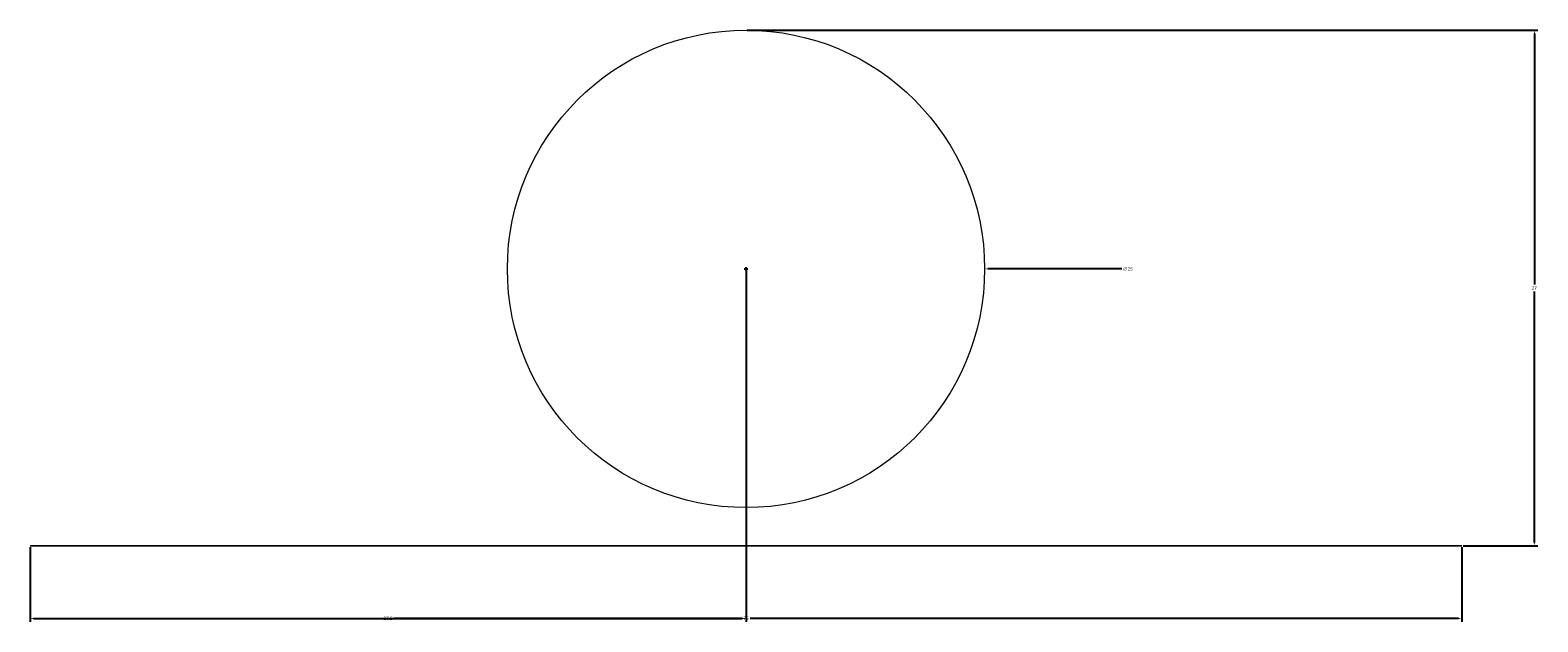
# Model space of a CAD drawing. Units: millimetres. Extents: x 326.6 to 405.6, y -4 to 27.
import ezdxf

# ---------------------------------------------------------------- set-up
doc = ezdxf.new("R2010")
doc.units = ezdxf.units.MM
doc.layers.add('M-CONS', color=8, linetype='Continuous', lineweight=13)
doc.layers.add('M-DIMS', color=2, linetype='Continuous', lineweight=18)
doc.styles.get("Standard").update_dxf_attribs({"font": 'arial.ttf'})
doc.dimstyles.get("Standard").update_dxf_attribs({"dimtxt": 0.18, "dimasz": 0.18, "dimexe": 0.18, "dimexo": 0.0625, "dimgap": 0.09, "dimtad": 0, "dimtih": 1, "dimtoh": 1, "dimdec": 4, "dimzin": 0, "dimdsep": 46, "dimtxsty": 'Standard', "dimcen": 0.09, "dimadec": 0, "dimazin": 0, "dimtfac": 1, "dimtdec": 4, "dimtofl": 0, "dimtmove": 0, "dimatfit": 3, "dimfxl": 1, "dimtolj": 1, "dimtzin": 0, "dimarcsym": 0})

# ---------------------------------------------------------------- blocks, each defined once
blk = doc.blocks.new('*D1')
at = {"layer": 'Defpoints', "color": 0, "transparency": 16777216}
for p in [(364.095, 14.5), (326.595, 0), (364.095, -3.8)]:
    blk.add_point(p, dxfattribs=at)
at = {"layer": 'M-DIMS', "color": 0, "lineweight": -2, "transparency": 16777216}
for p, q in [((364.095, 14.438), (364.095, -3.98)), ((326.595, -0.062), (326.595, -3.98)), ((326.775, -3.8), (345.021, -3.8)), ((363.915, -3.8), (345.67, -3.8))]:
    blk.add_line(p, q, dxfattribs=at)
at = {"layer": 'M-DIMS', "color": 0, "transparency": 16777216}
for points in [[(326.775, -3.77), (326.775, -3.83), (326.595, -3.8)], [(363.915, -3.77), (363.915, -3.83), (364.095, -3.8)]]:
    blk.add_solid(points, dxfattribs=at)
at = {"layer": 'M-DIMS', "color": 0, "transparency": 16777216, "insert": (345.345, -3.8), "char_height": 0.18, "attachment_point": 5}
blk.add_mtext('\\A1;37.5', dxfattribs=at)
blk = doc.blocks.new('*D2')
at = {"layer": 'Defpoints', "color": 0, "transparency": 16777216}
for p in [(326.595, 0), (401.595, 0), (401.595, -3.8)]:
    blk.add_point(p, dxfattribs=at)
at = {"layer": 'M-DIMS', "color": 0, "lineweight": -2, "transparency": 16777216}
for p, q in [((326.595, -0.062), (326.595, -3.98)), ((401.595, -0.062), (401.595, -3.98)), ((326.775, -3.8), (363.877, -3.8)), ((401.415, -3.8), (364.314, -3.8))]:
    blk.add_line(p, q, dxfattribs=at)
at = {"layer": 'M-DIMS', "color": 0, "transparency": 16777216}
for points in [[(326.775, -3.77), (326.775, -3.83), (326.595, -3.8)], [(401.415, -3.77), (401.415, -3.83), (401.595, -3.8)]]:
    blk.add_solid(points, dxfattribs=at)
at = {"layer": 'M-DIMS', "color": 0, "transparency": 16777216, "insert": (364.095, -3.8), "char_height": 0.18, "attachment_point": 5}
blk.add_mtext('\\A1;75', dxfattribs=at)
blk = doc.blocks.new('*D3')
at = {"layer": 'Defpoints', "color": 0, "transparency": 16777216}
for p in [(364.095, 27), (405.395, 27), (401.595, 0)]:
    blk.add_point(p, dxfattribs=at)
at = {"layer": 'M-DIMS', "color": 0, "lineweight": -2, "transparency": 16777216}
for p, q in [((364.158, 27), (405.575, 27)), ((405.395, 26.82), (405.395, 13.68)), ((405.395, 0.18), (405.395, 13.32)), ((401.658, 0), (405.575, 0))]:
    blk.add_line(p, q, dxfattribs=at)
at = {"layer": 'M-DIMS', "color": 0, "transparency": 16777216}
for points in [[(405.365, 26.82), (405.425, 26.82), (405.395, 27)], [(405.365, 0.18), (405.425, 0.18), (405.395, 0)]]:
    blk.add_solid(points, dxfattribs=at)
at = {"layer": 'M-DIMS', "color": 0, "transparency": 16777216, "insert": (405.395, 13.5), "char_height": 0.18, "attachment_point": 5}
blk.add_mtext('\\A1;27', dxfattribs=at)
blk = doc.blocks.new('*D4')
at = {"layer": 'Defpoints', "color": 0, "transparency": 16777216}
for p in [(351.595, 14.5), (376.595, 14.5)]:
    blk.add_point(p, dxfattribs=at)
at = {"layer": 'M-DIMS', "color": 0, "lineweight": -2, "transparency": 16777216}
for p, q in [((364.005, 14.5), (364.185, 14.5)), ((364.095, 14.41), (364.095, 14.59)), ((383.778, 14.5), (376.775, 14.5))]:
    blk.add_line(p, q, dxfattribs=at)
at = {"layer": 'M-DIMS', "color": 0, "transparency": 16777216}
blk.add_solid([(376.775, 14.53), (376.775, 14.47), (376.595, 14.5)], dxfattribs=at)
at = {"layer": 'M-DIMS', "color": 0, "transparency": 16777216, "insert": (384.095, 14.5), "char_height": 0.18, "attachment_point": 5}
blk.add_mtext('\\A1;∅25', dxfattribs=at)

msp = doc.modelspace()

# ---------------------------------------------------------------- linework, layer by layer
at = {"layer": 'M-CONS', "extrusion": (0, -1, 0)}
msp.add_lwpolyline([(326.595, 149.018), (401.595, 149.018), (401.595, 89.018), (381.595, 89.018), (381.595, 129.018), (346.595, 129.018), (346.595, 89.018), (326.595, 89.018)], close=True, dxfattribs=at)
at = {"layer": 'M-CONS'}
msp.add_circle((364.095, 14.5, 149.018), 12.5, dxfattribs=at)

# ---------------------------------------------------------------- dimensions: what is measured, and where the dimension line sits
at = {"layer": 'M-DIMS'}
dim = msp.add_linear_dim(base=(405.395, 27), p1=(401.595, 0), p2=(364.095, 27), angle=90, dimstyle='Standard', override={"dimdec": 0, "dimlfac": 1, "dimrnd": 0, "dimzin": 0, "dimdsep": 46, "dimlunit": 2}, dxfattribs=at)
dim.commit()
dim.dimension.update_dxf_attribs({"geometry": '*D3', "text_midpoint": (405.395, 13.5)})
for base, p2, override, picture, middle in [((364.095, -3.8), (364.095, 14.5), {"dimdec": 1, "dimlfac": 1, "dimrnd": 0, "dimzin": 0, "dimdsep": 46, "dimlunit": 2}, '*D1', (345.345, -3.8)), ((401.595, -3.8), (401.595, 0), {"dimdec": 0, "dimlfac": 1, "dimrnd": 0, "dimzin": 0, "dimdsep": 46, "dimlunit": 2}, '*D2', (364.095, -3.8))]:
    dim = msp.add_linear_dim(base=base, p1=(326.595, 0), p2=p2, dimstyle='Standard', override=override, dxfattribs=at)
    dim.commit()
    dim.dimension.update_dxf_attribs({"geometry": picture, "text_midpoint": middle})
dim = msp.add_diameter_dim_2p(p1=(351.595, 14.5), p2=(376.595, 14.5), dimstyle='Standard', override={"dimdec": 0, "dimlfac": 1, "dimrnd": 0, "dimzin": 0, "dimdsep": 46, "dimlunit": 2}, dxfattribs=at)
dim.commit()
dim.dimension.update_dxf_attribs({"geometry": '*D4', "text_midpoint": (384.095, 14.5), "dimtype": 163})

doc.saveas('drawing.dxf')
